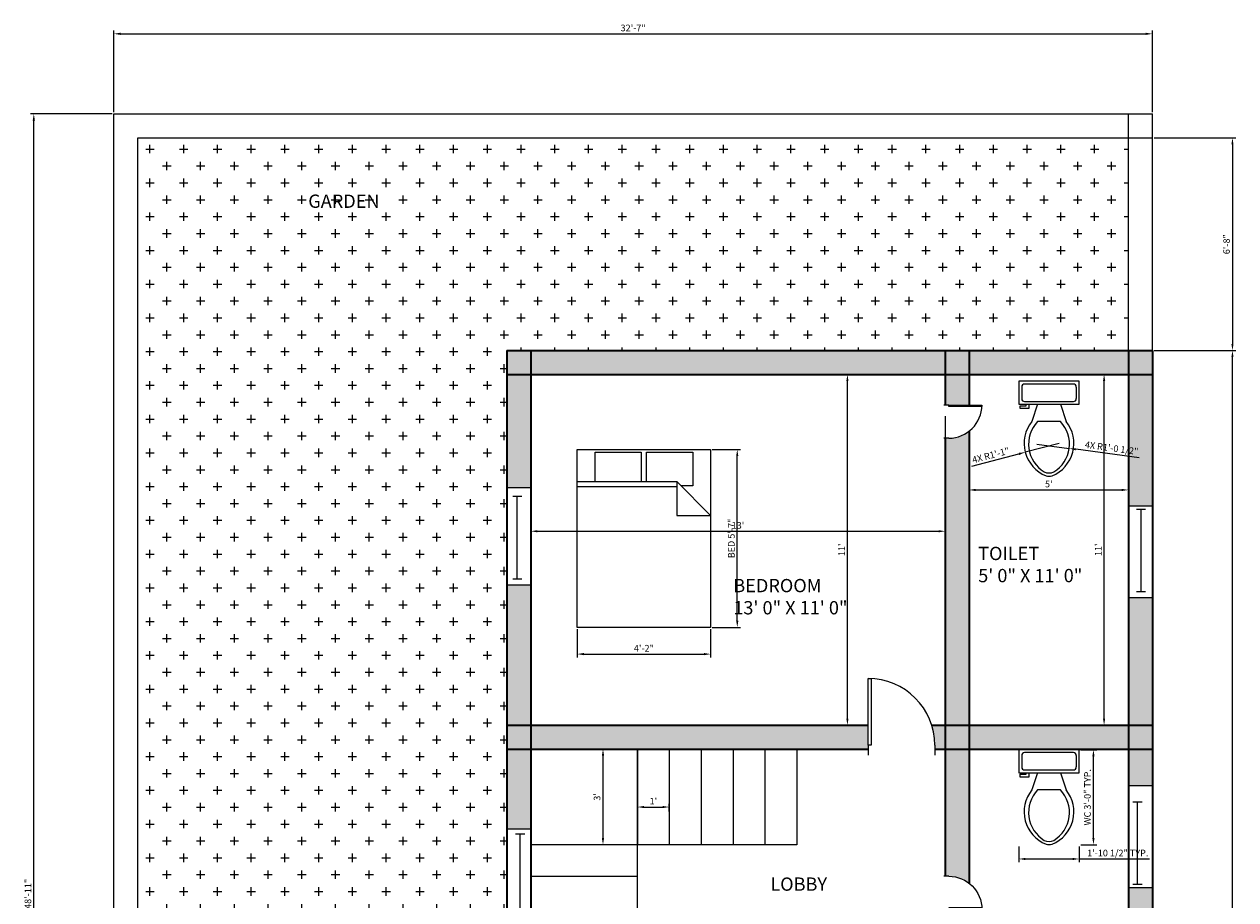
# Model space of a CAD drawing. Units: millimetres. Extents: x 2602 to 3574, y 848 to 1501.
# Tile 2 of 3: x 2602 to 3058, y 1172 to 1501. Entities that reach past the tile are written whole.
import ezdxf

# ---------------------------------------------------------------- set-up
doc = ezdxf.new("R2010")
doc.units = ezdxf.units.MM
for name, color, linetype, lineweight in [('A-ANNO-DIMS', 170, 'Continuous', 18), ('A-AREA-IDEN', 200, 'Continuous', 18), ('A-FLOR-FIXT', 90, 'Continuous', 18), ('A-WALL-PATT', 140, 'Continuous', 13), ('C-PROP', 140, 'Continuous', 25), ('doors', 10, 'Continuous', 25), ('furniture', 90, 'Continuous', 18), ('L-PLNT-PATT', 152, 'Continuous', 13), ('STAIRCASE', 30, 'Continuous', 25), ('walls', 140, 'Continuous', 35), ('windows', 40, 'Continuous', 18)]:
    doc.layers.add(name, color=color, linetype=linetype, lineweight=lineweight)
doc.styles.get("Standard").update_dxf_attribs({"font": 'arial.ttf'})
doc.dimstyles.new('ISO-25', dxfattribs={"dimtxt": 2.5, "dimasz": 2.5, "dimexe": 1.25, "dimexo": 0.625, "dimtad": 1, "dimdec": 0, "dimlunit": 3, "dimtxsty": 'Standard', "dimcen": 2.5, "dimadec": 0, "dimazin": 0, "dimtfac": 1, "dimtdec": 0, "dimtmove": 0, "dimatfit": 3, "dimfxl": 1, "dimarcsym": 0})

# ---------------------------------------------------------------- blocks, each defined once
blk = doc.blocks.new('*U2')
for p, q in [((0, 0), (0, -6)), ((40, 0), (40, -6))]:
    blk.add_line(p, q)
blk.add_lwpolyline([(0, 0), (0, 40), (1.75, 40), (1.75, 0)], close=True)
blk.add_arc((0, 0), 40, 0, 90)
blk = doc.blocks.new('*U4')
for p, q in [((0, 4), (0, 0)), ((0, 2), (36, 2)), ((36, 4), (36, 0))]:
    blk.add_line(p, q)
blk = doc.blocks.new('Bed - Queen')
for p, q in [((0, -80.00003), (0, 0)), ((0, 0), (59.99999, 0)), ((59.99999, 0), (59.99999, -80.00003)), ((7.99999, -1.2), (28.79998, -1.2)), ((7.99999, -14.4), (7.99999, -1.2)), ((28.79998, -1.2), (28.79998, -14.4)), ((31.19999, -1.2), (51.99999, -1.2)), ((31.19999, -14.4), (31.19999, -1.2)), ((51.99999, -1.2), (51.99999, -16.4)), ((0, -14.4), (44.8, -14.4)), ((59.99999, -29.6), (44.8, -14.4)), ((44.8, -14.4), (44.8, -29.6)), ((44.8, -16.8), (0, -16.8)), ((51.99999, -16.4), (46.79936, -16.4)), ((44.8, -29.6), (59.99999, -29.6)), ((59.99999, -80.00003), (0, -80.00003))]:
    blk.add_line(p, q)
blk = doc.blocks.new('Toilet - top')
for p, q in [((9.5, -6), (9.5, -2)), ((-8, -8.5), (-8, -8)), ((-7, -8), (-7, -9.5)), ((-4, -8), (-6, -14)), ((4, -8), (6, -14)), ((-10, -8.5), (-8, -8.5)), ((-10, -9.5), (-10, -8.5)), ((-7, -9.5), (-10, -9.5)), ((4, -14), (-4, -14))]:
    blk.add_line(p, q)
blk.add_lwpolyline([(10.5, -8), (10.5, 0), (-10.5, 0), (-10.5, -8)], close=True)
for points in [[(-9.5, -2), (-9.5, -6)], [(8.5, -1), (-8.5, -1)], [(-8.5, -7), (8.5, -7)]]:
    blk.add_lwpolyline(points)
for centre, radius, start, end in [((-8.62, -1.88), 0.884, 81.8699, 188.1301), ((8.62, -1.88), 0.884, 351.8699, 98.1301), ((-8.62, -6.12), 0.884, 171.8699, 278.1301), ((8.62, -6.12), 0.884, 261.8699, 8.1301), ((3.52, -21.58), 12.17, 141.4691, 247.9714), ((4.2, -21.82), 11.33, 136.3677, 238.9468), ((-3.52, -21.58), 12.17, 292.0284, 38.5307), ((-4.2, -21.82), 11.33, 301.053, 43.6321), ((0, -27.88), 4, 245.7318, 294.2682), ((0, -29), 4, 254.8605, 285.1395)]:
    blk.add_arc(centre, radius, start, end)
blk = doc.blocks.new('*D9')
at = {"layer": 'A-ANNO-DIMS', "color": 0, "lineweight": -2, "transparency": 16777216}
for p, q in [((2792.88, 1353.71), (2792.88, 1309.09)), ((2948.88, 1353.71), (2948.88, 1309.09)), ((2795.38, 1310.34), (2946.38, 1310.34))]:
    blk.add_line(p, q, dxfattribs=at)
at = {"layer": 'A-ANNO-DIMS', "color": 0, "transparency": 16777216}
for points in [[(2795.38, 1310.75), (2795.38, 1309.92), (2792.88, 1310.34)], [(2946.38, 1310.75), (2946.38, 1309.92), (2948.88, 1310.34)]]:
    blk.add_solid(points, dxfattribs=at)
at = {"layer": 'Defpoints', "color": 0, "transparency": 16777216}
for p in [(2792.88, 1354.34), (2948.88, 1354.34), (2948.88, 1310.34)]:
    blk.add_point(p, dxfattribs=at)
at = {"layer": 'A-ANNO-DIMS', "color": 0, "transparency": 16777216, "insert": (2870.88, 1312.24), "char_height": 2.5, "attachment_point": 5}
blk.add_mtext("13'", dxfattribs=at)
blk = doc.blocks.new('*D10')
at = {"layer": 'A-ANNO-DIMS', "color": 0, "lineweight": -2, "transparency": 16777216}
for p, q in [((2913.88, 1369.36), (2910.84, 1369.36)), ((2912.09, 1239.86), (2912.09, 1366.86)), ((2913.08, 1237.36), (2910.84, 1237.36))]:
    blk.add_line(p, q, dxfattribs=at)
at = {"layer": 'A-ANNO-DIMS', "color": 0, "transparency": 16777216}
for points in [[(2911.67, 1366.86), (2912.5, 1366.86), (2912.09, 1369.36)], [(2911.67, 1239.86), (2912.5, 1239.86), (2912.09, 1237.36)]]:
    blk.add_solid(points, dxfattribs=at)
at = {"layer": 'Defpoints', "color": 0, "transparency": 16777216}
for p in [(2912.09, 1369.36), (2914.5, 1369.36), (2913.71, 1237.36)]:
    blk.add_point(p, dxfattribs=at)
at = {"layer": 'A-ANNO-DIMS', "color": 0, "transparency": 16777216, "insert": (2910.21, 1303.36), "char_height": 2.5, "attachment_point": 5, "rotation": 90}
blk.add_mtext("11'", dxfattribs=at)
blk = doc.blocks.new('*D11')
at = {"layer": 'A-ANNO-DIMS', "color": 0, "lineweight": -2, "transparency": 16777216}
for p, q in [((2957.88, 1326.51), (2957.88, 1327.14)), ((2960.38, 1325.89), (3015.38, 1325.89)), ((3017.88, 1326.51), (3017.88, 1327.14))]:
    blk.add_line(p, q, dxfattribs=at)
at = {"layer": 'A-ANNO-DIMS', "color": 0, "transparency": 16777216}
for points in [[(2960.38, 1326.3), (2960.38, 1325.47), (2957.88, 1325.89)], [(3015.38, 1326.3), (3015.38, 1325.47), (3017.88, 1325.89)]]:
    blk.add_solid(points, dxfattribs=at)
at = {"layer": 'Defpoints', "color": 0, "transparency": 16777216}
for p in [(2957.88, 1325.89), (3017.88, 1325.89), (3017.88, 1325.89)]:
    blk.add_point(p, dxfattribs=at)
at = {"layer": 'A-ANNO-DIMS', "color": 0, "transparency": 16777216, "insert": (2987.88, 1327.78), "char_height": 2.5, "attachment_point": 5}
blk.add_mtext("5'", dxfattribs=at)
blk = doc.blocks.new('*D12')
at = {"layer": 'A-ANNO-DIMS', "color": 0, "lineweight": -2, "transparency": 16777216}
for p, q in [((3006.5, 1369.36), (3009.96, 1369.36)), ((3008.71, 1239.86), (3008.71, 1366.86)), ((3004.5, 1237.36), (3009.96, 1237.36))]:
    blk.add_line(p, q, dxfattribs=at)
at = {"layer": 'A-ANNO-DIMS', "color": 0, "transparency": 16777216}
for points in [[(3008.29, 1366.86), (3009.13, 1366.86), (3008.71, 1369.36)], [(3008.29, 1239.86), (3009.13, 1239.86), (3008.71, 1237.36)]]:
    blk.add_solid(points, dxfattribs=at)
at = {"layer": 'Defpoints', "color": 0, "transparency": 16777216}
for p in [(3005.87, 1369.36), (3008.71, 1369.36), (3003.87, 1237.36)]:
    blk.add_point(p, dxfattribs=at)
at = {"layer": 'A-ANNO-DIMS', "color": 0, "transparency": 16777216, "insert": (3006.83, 1303.36), "char_height": 2.5, "attachment_point": 5, "rotation": 90}
blk.add_mtext("11'", dxfattribs=at)
blk = doc.blocks.new('*D19')
at = {"layer": 'A-ANNO-DIMS', "color": 0, "lineweight": -2, "transparency": 16777216}
for p, q in [((2832.4, 1228.36), (2818.82, 1228.36)), ((2820.07, 1225.86), (2820.07, 1194.86)), ((2832.4, 1192.36), (2818.82, 1192.36))]:
    blk.add_line(p, q, dxfattribs=at)
at = {"layer": 'A-ANNO-DIMS', "color": 0, "transparency": 16777216}
for points in [[(2819.65, 1225.86), (2820.49, 1225.86), (2820.07, 1228.36)], [(2819.65, 1194.86), (2820.49, 1194.86), (2820.07, 1192.36)]]:
    blk.add_solid(points, dxfattribs=at)
at = {"layer": 'Defpoints', "color": 0, "transparency": 16777216}
for p in [(2833.03, 1228.36), (2820.07, 1192.36), (2833.03, 1192.36)]:
    blk.add_point(p, dxfattribs=at)
at = {"layer": 'A-ANNO-DIMS', "color": 0, "transparency": 16777216, "insert": (2818.17, 1210.36), "char_height": 2.5, "attachment_point": 5, "rotation": 90}
blk.add_mtext("3'", dxfattribs=at)
blk = doc.blocks.new('*D20')
at = {"layer": 'A-ANNO-DIMS', "color": 0, "lineweight": -2, "transparency": 16777216}
for p, q in [((2833.03, 1204.9), (2833.03, 1207.81)), ((2835.53, 1206.56), (2842.53, 1206.56)), ((2845.03, 1204.9), (2845.03, 1207.81))]:
    blk.add_line(p, q, dxfattribs=at)
at = {"layer": 'A-ANNO-DIMS', "color": 0, "transparency": 16777216}
for points in [[(2835.53, 1206.97), (2835.53, 1206.14), (2833.03, 1206.56)], [(2842.53, 1206.97), (2842.53, 1206.14), (2845.03, 1206.56)]]:
    blk.add_solid(points, dxfattribs=at)
at = {"layer": 'Defpoints', "color": 0, "transparency": 16777216}
for p in [(2833.03, 1204.28), (2845.03, 1206.56), (2845.03, 1204.28)]:
    blk.add_point(p, dxfattribs=at)
at = {"layer": 'A-ANNO-DIMS', "color": 0, "transparency": 16777216, "insert": (2839.03, 1208.44), "char_height": 2.5, "attachment_point": 5}
blk.add_mtext("1'", dxfattribs=at)
blk = doc.blocks.new('*D28')
at = {"layer": 'A-ANNO-DIMS', "color": 0, "lineweight": -2, "transparency": 16777216}
for p, q in [((2999.96, 1228.12), (3005.95, 1228.12)), ((3004.7, 1194.87), (3004.7, 1225.62)), ((2999.96, 1192.37), (3005.95, 1192.37))]:
    blk.add_line(p, q, dxfattribs=at)
at = {"layer": 'A-ANNO-DIMS', "color": 0, "transparency": 16777216}
for points in [[(3004.28, 1225.62), (3005.12, 1225.62), (3004.7, 1228.12)], [(3004.28, 1194.87), (3005.12, 1194.87), (3004.7, 1192.37)]]:
    blk.add_solid(points, dxfattribs=at)
at = {"layer": 'Defpoints', "color": 0, "transparency": 16777216}
for p in [(2999.34, 1228.12), (3004.7, 1228.12), (2999.34, 1192.37)]:
    blk.add_point(p, dxfattribs=at)
at = {"layer": 'A-ANNO-DIMS', "color": 0, "transparency": 16777216, "insert": (3002.78, 1210.24), "char_height": 2.5, "attachment_point": 5, "rotation": 90}
blk.add_mtext('WC 3\'-0" TYP.', dxfattribs=at)
blk = doc.blocks.new('*D29')
at = {"layer": 'A-ANNO-DIMS', "color": 0, "lineweight": -2, "transparency": 16777216}
for p, q in [((2976.61, 1191.74), (2976.61, 1185.75)), ((2999.34, 1191.74), (2999.34, 1185.75)), ((2979.11, 1187), (2996.84, 1187)), ((2999.34, 1187), (3025.86, 1187))]:
    blk.add_line(p, q, dxfattribs=at)
at = {"layer": 'A-ANNO-DIMS', "color": 0, "transparency": 16777216}
for points in [[(2979.11, 1187.42), (2979.11, 1186.59), (2976.61, 1187)], [(2996.84, 1187.42), (2996.84, 1186.59), (2999.34, 1187)]]:
    blk.add_solid(points, dxfattribs=at)
at = {"layer": 'Defpoints', "color": 0, "transparency": 16777216}
for p in [(2976.61, 1192.37), (2999.34, 1192.37), (2999.34, 1187)]:
    blk.add_point(p, dxfattribs=at)
at = {"layer": 'A-ANNO-DIMS', "color": 0, "transparency": 16777216, "insert": (3013.85, 1188.92), "char_height": 2.5, "attachment_point": 5}
blk.add_mtext('1\'-10 1/2" TYP.', dxfattribs=at)
blk = doc.blocks.new('*D32')
at = {"layer": 'A-ANNO-DIMS', "color": 0, "lineweight": -2, "transparency": 16777216}
for p, q in [((2861.2, 1341.1), (2871.87, 1341.1)), ((2870.62, 1276.65), (2870.62, 1338.6)), ((2861.2, 1274.15), (2871.87, 1274.15))]:
    blk.add_line(p, q, dxfattribs=at)
at = {"layer": 'A-ANNO-DIMS', "color": 0, "transparency": 16777216}
for points in [[(2870.2, 1338.6), (2871.04, 1338.6), (2870.62, 1341.1)], [(2870.2, 1276.65), (2871.04, 1276.65), (2870.62, 1274.15)]]:
    blk.add_solid(points, dxfattribs=at)
at = {"layer": 'Defpoints', "color": 0, "transparency": 16777216}
for p in [(2860.58, 1341.1), (2870.62, 1341.1), (2860.58, 1274.15)]:
    blk.add_point(p, dxfattribs=at)
at = {"layer": 'A-ANNO-DIMS', "color": 0, "transparency": 16777216, "insert": (2868.72, 1307.63), "char_height": 2.5, "attachment_point": 5, "rotation": 90}
blk.add_mtext('BED 5\'-7"', dxfattribs=at)
blk = doc.blocks.new('*D33')
at = {"layer": 'A-ANNO-DIMS', "color": 0, "lineweight": -2, "transparency": 16777216}
for p, q in [((2810.37, 1273.53), (2810.37, 1262.86)), ((2860.58, 1273.53), (2860.58, 1262.86)), ((2812.87, 1264.11), (2858.08, 1264.11))]:
    blk.add_line(p, q, dxfattribs=at)
at = {"layer": 'A-ANNO-DIMS', "color": 0, "transparency": 16777216}
for points in [[(2812.87, 1264.53), (2812.87, 1263.69), (2810.37, 1264.11)], [(2858.08, 1264.53), (2858.08, 1263.69), (2860.58, 1264.11)]]:
    blk.add_solid(points, dxfattribs=at)
at = {"layer": 'Defpoints', "color": 0, "transparency": 16777216}
for p in [(2810.37, 1274.15), (2860.58, 1274.15), (2860.58, 1264.11)]:
    blk.add_point(p, dxfattribs=at)
at = {"layer": 'A-ANNO-DIMS', "color": 0, "transparency": 16777216, "insert": (2835.47, 1265.99), "char_height": 2.5, "attachment_point": 5}
blk.add_mtext('4\'-2"', dxfattribs=at)
blk = doc.blocks.new('*D40')
at = {"layer": 'A-ANNO-DIMS', "color": 0, "lineweight": -2, "transparency": 16777216}
for p, q in [((2635.95, 1468.01), (2635.95, 1498.79)), ((2638.45, 1497.54), (3024.38, 1497.54)), ((3026.88, 1468.01), (3026.88, 1498.79))]:
    blk.add_line(p, q, dxfattribs=at)
at = {"layer": 'A-ANNO-DIMS', "color": 0, "transparency": 16777216}
for points in [[(2638.45, 1497.96), (2638.45, 1497.12), (2635.95, 1497.54)], [(3024.38, 1497.96), (3024.38, 1497.12), (3026.88, 1497.54)]]:
    blk.add_solid(points, dxfattribs=at)
at = {"layer": 'Defpoints', "color": 0, "transparency": 16777216}
for p in [(3026.88, 1497.54), (2635.95, 1467.39), (3026.88, 1467.39)]:
    blk.add_point(p, dxfattribs=at)
at = {"layer": 'A-ANNO-DIMS', "color": 0, "transparency": 16777216, "insert": (2831.42, 1499.44), "char_height": 2.5, "attachment_point": 5}
blk.add_mtext('32\'-7"', dxfattribs=at)
blk = doc.blocks.new('*D41')
at = {"layer": 'A-ANNO-DIMS', "color": 0, "lineweight": -2, "transparency": 16777216}
for p, q in [((2635.33, 1467.39), (2604.55, 1467.39)), ((2605.8, 882.86), (2605.8, 1464.89)), ((2635.33, 880.36), (2604.55, 880.36))]:
    blk.add_line(p, q, dxfattribs=at)
at = {"layer": 'A-ANNO-DIMS', "color": 0, "transparency": 16777216}
for points in [[(2605.39, 1464.89), (2606.22, 1464.89), (2605.8, 1467.39)], [(2605.39, 882.86), (2606.22, 882.86), (2605.8, 880.36)]]:
    blk.add_solid(points, dxfattribs=at)
at = {"layer": 'Defpoints', "color": 0, "transparency": 16777216}
for p in [(2605.8, 1467.39), (2635.95, 1467.39), (2635.95, 880.36)]:
    blk.add_point(p, dxfattribs=at)
at = {"layer": 'A-ANNO-DIMS', "color": 0, "transparency": 16777216, "insert": (2603.9, 1173.88), "char_height": 2.5, "attachment_point": 5, "rotation": 90}
blk.add_mtext('48\'-11"', dxfattribs=at)
blk = doc.blocks.new('*D42')
at = {"layer": 'A-ANNO-DIMS', "color": 0, "lineweight": -2, "transparency": 16777216}
for p, q in [((3027.5, 1378.36), (3058.28, 1378.36)), ((3057.03, 891.86), (3057.03, 1375.86)), ((3027.5, 889.36), (3058.28, 889.36))]:
    blk.add_line(p, q, dxfattribs=at)
at = {"layer": 'A-ANNO-DIMS', "color": 0, "transparency": 16777216}
for points in [[(3056.61, 1375.86), (3057.44, 1375.86), (3057.03, 1378.36)], [(3056.61, 891.86), (3057.44, 891.86), (3057.03, 889.36)]]:
    blk.add_solid(points, dxfattribs=at)
at = {"layer": 'Defpoints', "color": 0, "transparency": 16777216}
for p in [(3026.88, 1378.36), (3057.03, 1378.36), (3026.88, 889.36)]:
    blk.add_point(p, dxfattribs=at)
at = {"layer": 'A-ANNO-DIMS', "color": 0, "transparency": 16777216, "insert": (3055.12, 1133.86), "char_height": 2.5, "attachment_point": 5, "rotation": 90}
blk.add_mtext('40\'-9"', dxfattribs=at)
blk = doc.blocks.new('*D43')
at = {"layer": 'A-ANNO-DIMS', "color": 0, "lineweight": -2, "transparency": 16777216}
for p, q in [((3027.5, 1458.39), (3058.28, 1458.39)), ((3057.03, 1455.89), (3057.03, 1380.86)), ((3027.5, 1378.36), (3058.28, 1378.36))]:
    blk.add_line(p, q, dxfattribs=at)
at = {"layer": 'A-ANNO-DIMS', "color": 0, "transparency": 16777216}
for points in [[(3056.61, 1455.89), (3057.44, 1455.89), (3057.03, 1458.39)], [(3056.61, 1380.86), (3057.44, 1380.86), (3057.03, 1378.36)]]:
    blk.add_solid(points, dxfattribs=at)
at = {"layer": 'Defpoints', "color": 0, "transparency": 16777216}
for p in [(3026.88, 1458.39), (3026.88, 1378.36), (3057.03, 1378.36)]:
    blk.add_point(p, dxfattribs=at)
at = {"layer": 'A-ANNO-DIMS', "color": 0, "transparency": 16777216, "insert": (3055.12, 1418.37), "char_height": 2.5, "attachment_point": 5, "rotation": 90}
blk.add_mtext('6\'-8"', dxfattribs=at)
blk = doc.blocks.new('*D59')
at = {"layer": 'A-ANNO-DIMS', "color": 0, "lineweight": -2, "transparency": 16777216}
for p, q in [((2991.78, 1343.42), (2979.05, 1340.08)), ((2958.97, 1334.8), (2976.63, 1339.44))]:
    blk.add_line(p, q, dxfattribs=at)
at = {"layer": 'A-ANNO-DIMS', "color": 0, "transparency": 16777216}
blk.add_solid([(2976.53, 1339.84), (2976.74, 1339.04), (2979.05, 1340.08)], dxfattribs=at)
at = {"layer": 'Defpoints', "color": 0, "transparency": 16777216}
for p in [(2991.78, 1343.42), (2979.05, 1340.08)]:
    blk.add_point(p, dxfattribs=at)
at = {"layer": 'A-ANNO-DIMS', "color": 0, "transparency": 16777216, "insert": (2966.11, 1338.62), "char_height": 2.5, "attachment_point": 5, "rotation": 14.7194}
blk.add_mtext('4X R1\'-1"', dxfattribs=at)
blk = doc.blocks.new('*D60')
at = {"layer": 'A-ANNO-DIMS', "color": 0, "lineweight": -2, "transparency": 16777216}
for p, q in [((2983.43, 1343.17), (2995.58, 1341.53)), ((3021.93, 1337.99), (2998.06, 1341.2))]:
    blk.add_line(p, q, dxfattribs=at)
at = {"layer": 'A-ANNO-DIMS', "color": 0, "transparency": 16777216}
blk.add_solid([(2998.11, 1341.61), (2998, 1340.79), (2995.58, 1341.53)], dxfattribs=at)
at = {"layer": 'Defpoints', "color": 0, "transparency": 16777216}
for p in [(2983.43, 1343.17), (2995.58, 1341.53)]:
    blk.add_point(p, dxfattribs=at)
at = {"layer": 'A-ANNO-DIMS', "color": 0, "transparency": 16777216, "insert": (3011.49, 1341.33), "char_height": 2.5, "attachment_point": 5, "rotation": 352.3431}
blk.add_mtext('4X R1\'-0 1/2"', dxfattribs=at)

msp = doc.modelspace()

# ---------------------------------------------------------------- hatches: boundary and pattern name
at = {"layer": 'A-WALL-PATT'}
h = msp.add_hatch(color=256, dxfattribs=at)
h.dxf.hatch_style = 1
h.paths.add_polyline_path([(2792.88, 1117.36), (2783.88, 1117.36), (2783.88, 1012.52), (2792.88, 1012.52)])
h.paths.add_polyline_path([(2957.88, 1117.36), (2948.88, 1117.36), (2948.88, 1057.36), (2957.88, 1057.36)])
h.paths.add_polyline_path([(2957.88, 1057.36), (2948.88, 1057.36), (2948.88, 1048.36), (2957.88, 1048.36)])
h.paths.add_polyline_path([(3002.51, 1057.36), (2957.88, 1057.36), (2957.88, 1048.36), (2999.91, 1048.36), (2999.91, 1049.72, -0.166059)])
h.paths.add_polyline_path([(3026.88, 1057.36), (3017.88, 1057.36), (3017.88, 1048.36), (3026.88, 1048.36)])
h.paths.add_polyline_path([(3017.88, 1057.36), (3012.39, 1057.36), (3012.39, 1049.72), (3012.39, 1048.36), (3017.88, 1048.36)])
h.paths.add_polyline_path([(3026.88, 1048.36), (3017.88, 1048.36), (3017.88, 1004.59), (3026.88, 1004.59)])
h.paths.add_polyline_path([(3026.88, 1069.96), (3017.88, 1069.96), (3017.88, 1057.36), (3026.88, 1057.36)])
h.paths.add_polyline_path([(3017.88, 1126.36), (2957.88, 1126.36), (2957.88, 1117.36), (3017.88, 1117.36)])
h.paths.add_polyline_path([(2957.88, 1126.36), (2948.88, 1126.36), (2948.88, 1117.36), (2957.88, 1117.36)])
h.paths.add_polyline_path([(2948.88, 1126.36), (2792.88, 1126.36), (2792.88, 1117.36), (2948.88, 1117.36)])
h.paths.add_polyline_path([(2957.88, 1168.02), (2950.23, 1168.02), (2948.88, 1168.02), (2948.88, 1126.36), (2957.88, 1126.36)])
h.paths.add_polyline_path([(3026.88, 1176.14), (3017.88, 1176.14), (3017.88, 1126.36), (3026.88, 1126.36)])
h.paths.add_polyline_path([(3026.88, 1126.36), (3017.88, 1126.36), (3017.88, 1117.36), (3026.88, 1117.36)])
h.paths.add_polyline_path([(3026.88, 1117.36), (3017.88, 1117.36), (3017.88, 1106.26), (3026.88, 1106.26)])
h.paths.add_polyline_path([(2792.88, 1163.71), (2783.88, 1163.71), (2783.88, 1126.36), (2792.88, 1126.36)])
h.paths.add_polyline_path([(2792.88, 1126.36), (2783.88, 1126.36), (2783.88, 1117.36), (2792.88, 1117.36)])
h.paths.add_polyline_path([(2921.88, 991.95), (2912.88, 991.95), (2912.88, 898.36), (2921.88, 898.36)])
h.paths.add_polyline_path([(3026.88, 966.36), (3017.88, 966.36), (3017.88, 898.36), (3026.88, 898.36)])
h.paths.add_polyline_path([(2792.88, 977.5), (2783.88, 977.5), (2783.88, 898.36), (2792.88, 898.36)])
h.paths.add_polyline_path([(2792.88, 1228.36), (2783.88, 1228.36), (2783.88, 1198.24), (2792.88, 1198.24)])
h.paths.add_polyline_path([(2792.88, 1290.09), (2783.88, 1290.09), (2783.88, 1237.36), (2792.88, 1237.36)])
h.paths.add_polyline_path([(2792.88, 1237.36), (2783.88, 1237.36), (2783.88, 1228.36), (2792.88, 1228.36)])
h.paths.add_polyline_path([(2948.88, 1378.36), (2792.88, 1378.36), (2792.88, 1369.36), (2948.88, 1369.36)])
h.paths.add_polyline_path([(2792.88, 1378.36), (2783.88, 1378.36), (2783.88, 1369.36), (2792.88, 1369.36)])
h.paths.add_polyline_path([(2792.88, 1369.36), (2783.88, 1369.36), (2783.88, 1326.82), (2792.88, 1326.82)])
h.paths.add_polyline_path([(2957.88, 1347.96, -0.166257), (2950.23, 1345.35), (2948.88, 1345.35), (2948.88, 1237.36), (2957.88, 1237.36)])
h.paths.add_polyline_path([(3017.88, 1237.36), (2957.88, 1237.36), (2957.88, 1228.36), (3017.88, 1228.36)])
h.paths.add_polyline_path([(2957.88, 1237.36), (2948.88, 1237.36), (2948.88, 1228.36), (2957.88, 1228.36)])
h.paths.add_polyline_path([(2948.88, 1237.36), (2943.82, 1237.36, -0.076419), (2944.98, 1229.83), (2944.98, 1228.36), (2948.88, 1228.36)])
h.paths.add_polyline_path([(3026.88, 1237.36), (3017.88, 1237.36), (3017.88, 1228.36), (3026.88, 1228.36)])
h.paths.add_polyline_path([(3026.88, 1285.23), (3017.88, 1285.23), (3017.88, 1237.36), (3026.88, 1237.36)])
h.paths.add_polyline_path([(3026.88, 1228.36), (3017.88, 1228.36), (3017.88, 1214.51), (3026.88, 1214.51)])
h.paths.add_polyline_path([(2919.9, 1237.36), (2792.88, 1237.36), (2792.88, 1228.36), (2919.9, 1228.36), (2919.9, 1229.83)])
h.paths.add_polyline_path([(2957.88, 1228.36), (2948.88, 1228.36), (2948.88, 1180.5), (2950.23, 1180.5, -0.166257), (2957.88, 1177.89)])
h.paths.add_polyline_path([(3026.88, 1369.36), (3017.88, 1369.36), (3017.88, 1319.81), (3026.88, 1319.81)])
h.paths.add_polyline_path([(3026.88, 1378.36), (3017.88, 1378.36), (3017.88, 1369.36), (3026.88, 1369.36)])
h.paths.add_polyline_path([(3017.88, 1378.36), (2957.88, 1378.36), (2957.88, 1369.36), (3017.88, 1369.36)])
h.paths.add_polyline_path([(2957.88, 1378.36), (2948.88, 1378.36), (2948.88, 1369.36), (2957.88, 1369.36)])
h.paths.add_polyline_path([(2957.88, 1369.36), (2948.88, 1369.36), (2948.88, 1357.83), (2950.23, 1357.83), (2957.88, 1357.83)])
at = {"layer": 'L-PLNT-PATT'}
h = msp.add_hatch(dxfattribs=at)
h.set_pattern_fill('CROSS', color=256)
h.paths.add_polyline_path([(3017.88, 1458.39), (2644.95, 1458.39), (2644.95, 1117.36), (2783.88, 1117.36), (2783.88, 1378.36), (3017.88, 1378.36)])

# ---------------------------------------------------------------- linework, layer by layer
at = {"layer": 'C-PROP'}
for p, q in [((3017.88, 1378.36), (3017.88, 1467.39)), ((3026.88, 1378.36), (3026.88, 1467.39))]:
    msp.add_line(p, q, dxfattribs=at)
for points in [[(2796.6, 880.36), (2635.95, 880.36), (2635.95, 1467.39), (3026.88, 1467.39)], [(2796.6, 889.36), (2644.95, 889.36), (2644.95, 1458.39), (3026.88, 1458.39)]]:
    msp.add_lwpolyline(points, dxfattribs=at)
at = {"layer": 'STAIRCASE'}
for p, q in [((2833.03, 1126.36), (2833.03, 1228.36)), ((2833.03, 1228.36), (2833.03, 1192.36)), ((2845.03, 1228.36), (2845.03, 1192.36)), ((2857.03, 1228.36), (2857.03, 1192.36)), ((2869.03, 1228.36), (2869.03, 1192.36)), ((2881.03, 1228.36), (2881.03, 1192.36)), ((2893.03, 1228.36), (2893.03, 1192.36)), ((2893.03, 1192.36), (2792.88, 1192.36)), ((2833.03, 1180.36), (2792.88, 1180.36))]:
    msp.add_line(p, q, dxfattribs=at)
at = {"layer": 'walls'}
for p, q in [((2783.88, 1378.36), (2783.88, 898.36)), ((2783.88, 1378.36), (3026.88, 1378.36)), ((2792.88, 1378.36), (2792.88, 898.36)), ((2948.88, 1378.36), (2948.88, 1357.83)), ((2957.88, 1378.36), (2957.88, 1357.83)), ((3017.88, 1378.36), (3017.88, 889.36)), ((3026.88, 1378.36), (3026.88, 889.36)), ((2783.88, 1369.36), (3026.88, 1369.36)), ((2957.88, 1347.96), (2957.88, 1177.89)), ((2948.88, 1345.35), (2948.88, 1180.5)), ((2783.88, 1237.36), (2919.9, 1237.36)), ((2943.82, 1237.36), (3026.88, 1237.36)), ((2783.88, 1228.36), (2919.9, 1228.36)), ((2944.98, 1228.36), (3026.88, 1228.36))]:
    msp.add_line(p, q, dxfattribs=at)
msp.add_lwpolyline([(3026.88, 1378.36), (3026.88, 889.36), (2821.68, 889.36)], dxfattribs=at)
at = {"layer": 'windows'}
for p, q in [((2783.88, 1326.82), (2792.88, 1326.82)), ((3026.88, 1319.81), (3017.88, 1319.81)), ((2792.88, 1290.09), (2783.88, 1290.09)), ((3026.88, 1285.23), (3017.88, 1285.23)), ((3026.88, 1214.51), (3017.88, 1214.51)), ((2792.88, 1198.24), (2783.88, 1198.24)), ((3026.88, 1176.14), (3017.88, 1176.14))]:
    msp.add_line(p, q, dxfattribs=at)

# ---------------------------------------------------------------- block references
at = {"layer": 'A-FLOR-FIXT', "xscale": 1.082000375667574, "yscale": 1.082000375667574, "zscale": 1.082000375667574}
for p in [(2987.98, 1366.77), (2987.98, 1228.12)]:
    msp.add_blockref('Toilet - top', p, dxfattribs=at)
at = {"layer": 'doors', "yscale": 0.3120057346177813, "zscale": 0.3120057346177813, "rotation": 270}
for p, xscale in [((2950.23, 1357.83), 0.3120057346177813), ((2950.23, 1168.02), -0.3120057346177813)]:
    msp.add_blockref('*U2', p, dxfattribs=dict(at, xscale=xscale))
at = {"layer": 'doors', "xscale": 0.6269655396628341, "yscale": 0.6269655396628341, "zscale": 0.6269655396628341}
msp.add_blockref('*U2', (2919.9, 1229.83), dxfattribs=at)
at = {"layer": 'furniture', "xscale": 0.8368204513331357, "yscale": 0.8368204513331357, "zscale": 0.8368204513331357}
msp.add_blockref('Bed - Queen', (2810.37, 1341.1), dxfattribs=at)
at = {"layer": 'windows', "xscale": 0.8623741926751115, "yscale": 0.8623741926751115, "zscale": 0.8623741926751115, "rotation": 90}
for p in [(2789.52, 1292.47), (3024.34, 1287.64), (3023, 1177.53), (2790.62, 1165.47)]:
    msp.add_blockref('*U4', p, dxfattribs=at)

# ---------------------------------------------------------------- texts
at = {"layer": 'A-AREA-IDEN', "char_height": 5, "attachment_point": 1}
for s, width, insert in [('GARDEN', 78.8471, (2709.12, 1437.05)), ('TOILET \\P5\' 0" X 11\' 0"', 51.6959, (2961.32, 1304.49)), ('BEDROOM \\P13\' 0" X 11\' 0"', 70.2503, (2869.13, 1292.39)), ('LOBBY', 41.8471, (2883.07, 1180.05))]:
    msp.add_mtext_dynamic_manual_height_columns(s, width=width, gutter_width=12.5, heights=[0], dxfattribs=dict(at, insert=insert))

# ---------------------------------------------------------------- dimensions: what is measured, and where the dimension line sits
at = {"layer": 'A-ANNO-DIMS'}
for base, p1, p2, override, picture, middle in [((3026.88, 1497.54), (2635.95, 1467.39), (3026.88, 1467.39), {"dimdec": 1, "dimlfac": 1, "dimrnd": 0, "dimzin": 1, "dimdsep": 46, "dimlunit": 4, "dimfrac": 2}, '*D40', (2831.42, 1499.44)), ((2948.88, 1310.34), (2792.88, 1354.34), (2948.88, 1354.34), {"dimclrd": 0, "dimclre": 0, "dimclrt": 0}, '*D9', (2870.88, 1312.24)), ((3017.88, 1325.89), (2957.88, 1325.89), (3017.88, 1325.89), {"dimclrd": 0, "dimclre": 0, "dimclrt": 0}, '*D11', (2987.88, 1327.78)), ((2860.58, 1264.11), (2810.37, 1274.15), (2860.58, 1274.15), {"dimdec": 1, "dimlfac": 1, "dimrnd": 0, "dimzin": 1, "dimdsep": 46, "dimlunit": 4, "dimfrac": 2}, '*D33', (2835.47, 1265.99)), ((2845.03, 1206.56), (2833.03, 1204.28), (2845.03, 1204.28), {"dimclrd": 0, "dimclre": 0, "dimclrt": 0}, '*D20', (2839.03, 1208.44))]:
    dim = msp.add_linear_dim(base=base, p1=p1, p2=p2, dimstyle='ISO-25', override=override, dxfattribs=at)
    dim.commit()
    dim.dimension.update_dxf_attribs({"geometry": picture, "text_midpoint": middle})
for base, p1, p2, override, picture, middle in [((2605.8, 1467.39), (2635.95, 880.36), (2635.95, 1467.39), {"dimdec": 1, "dimlfac": 1, "dimrnd": 0, "dimzin": 1, "dimdsep": 46, "dimlunit": 4, "dimfrac": 2}, '*D41', (2603.9, 1173.88)), ((3057.03, 1378.36), (3026.88, 1458.39), (3026.88, 1378.36), {"dimdec": 1, "dimlfac": 1, "dimrnd": 0, "dimzin": 1, "dimdsep": 46, "dimlunit": 4, "dimfrac": 2}, '*D43', (3055.12, 1418.37)), ((3057.03, 1378.36), (3026.88, 889.36), (3026.88, 1378.36), {"dimdec": 1, "dimlfac": 1, "dimrnd": 0, "dimzin": 1, "dimdsep": 46, "dimlunit": 4, "dimfrac": 2}, '*D42', (3055.12, 1133.86)), ((2912.09, 1369.36), (2913.71, 1237.36), (2914.5, 1369.36), {"dimclrd": 0, "dimclre": 0, "dimclrt": 0}, '*D10', (2910.21, 1303.36)), ((3008.71, 1369.36), (3003.87, 1237.36), (3005.87, 1369.36), {"dimclrd": 0, "dimclre": 0, "dimclrt": 0}, '*D12', (3006.83, 1303.36)), ((2820.07, 1192.36), (2833.03, 1228.36), (2833.03, 1192.36), {"dimclrd": 0, "dimclre": 0, "dimclrt": 0}, '*D19', (2818.17, 1210.36))]:
    dim = msp.add_linear_dim(base=base, p1=p1, p2=p2, angle=90, dimstyle='ISO-25', override=override, dxfattribs=at)
    dim.commit()
    dim.dimension.update_dxf_attribs({"geometry": picture, "text_midpoint": middle})
for center, mpoint, picture, middle in [((2983.43, 1343.17), (2995.58, 1341.53), '*D60', (3011.49, 1341.33)), ((2991.78, 1343.42), (2979.05, 1340.08), '*D59', (2966.11, 1338.62))]:
    dim = msp.add_radius_dim(center=center, mpoint=mpoint, text='4X <>', dimstyle='ISO-25', override={"dimdec": 1, "dimlfac": 1, "dimrnd": 0, "dimzin": 1, "dimdsep": 46, "dimlunit": 4, "dimfrac": 2}, dxfattribs=at)
    dim.commit()
    dim.dimension.update_dxf_attribs({"geometry": picture, "text_midpoint": middle})
for base, p1, p2, text, picture, middle in [((2870.6202, 1341.099), (2860.5784, 1274.1533), (2860.5784, 1341.099), 'BED <>', '*D32', (2868.7239, 1307.6261)), ((3004.7002, 1228.1218), (2999.3368, 1192.3658), (2999.3368, 1228.1218), 'WC <> TYP.', '*D28', (3002.7817, 1210.2438))]:
    dim = msp.add_linear_dim(base=base, p1=p1, p2=p2, angle=90, text=text, dimstyle='ISO-25', override={"dimdec": 1, "dimlfac": 1, "dimrnd": 0, "dimzin": 1, "dimdsep": 46, "dimlunit": 4, "dimfrac": 2}, dxfattribs=at)
    dim.commit()
    dim.dimension.update_dxf_attribs({"geometry": picture, "text_midpoint": middle})
dim = msp.add_linear_dim(base=(2999.34, 1187), p1=(2976.61, 1192.37), p2=(2999.34, 1192.37), text='<> TYP.', dimstyle='ISO-25', override={"dimdec": 1, "dimlfac": 1, "dimrnd": 0, "dimzin": 1, "dimdsep": 46, "dimlunit": 4, "dimfrac": 2}, dxfattribs=at)
dim.commit()
dim.dimension.update_dxf_attribs({"geometry": '*D29', "text_midpoint": (3013.85, 1188.92)})

doc.saveas('drawing.dxf')
